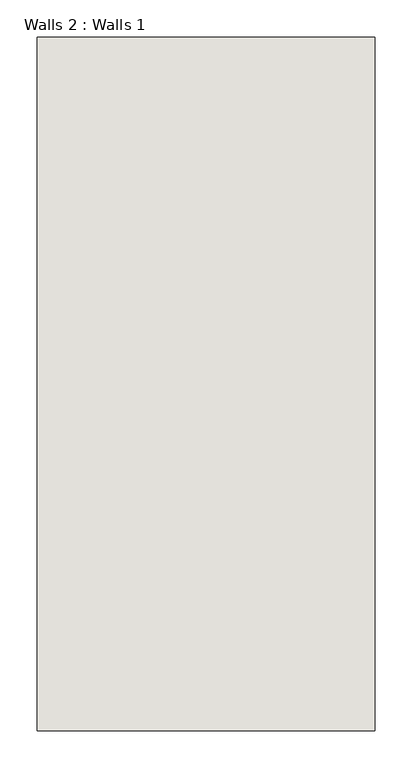
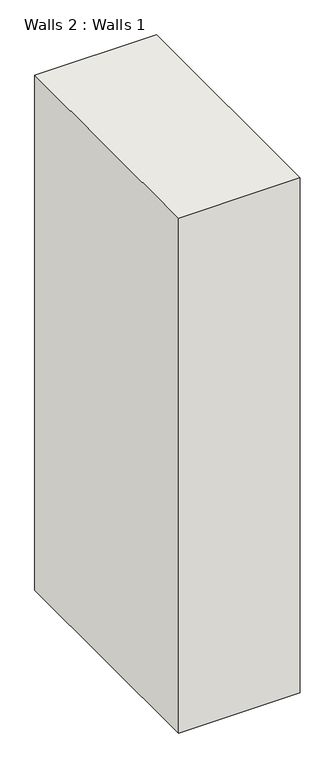
"""IFC4 building model written with IfcOpenShell, lengths in millimetres: wall geometry, Walls 2 : Walls 1."""

from ifc_helpers import new_model, si_unit, frame, origin, place, context, project, spatial, polyline, outline, extrude, faceted_brep, source, transform, mapped, element, save


def walls_2_walls_1_3d7729ba(model_context):
    return source(origin(), model_context, "Body", "SolidModel", [
        extrude(outline(polyline([(-8853.7371236, -1272.981648), (-8853.7371236, -2149.281648), (-9260.1371236, -2149.281648), (-9260.1371236, -1272.981648), (-8853.7371236, -1272.981648)])), frame((0.0, 0.0, 3775.1757913), z_axis=(0.0, 0.0, 1.0), x_axis=(1.0, 0.0, 0.0)), (0.0, 0.0, 1.0), 31.75),
        faceted_brep([(-8853.7371236, -1237.4497499, 5399.0952722), (-8853.7371236, -2174.681648, 5399.0952722), (-8853.7371236, -2174.681648, 3352.8), (-8853.7371236, -1237.4497499, 3352.8), (-8853.7371236, -1262.8497499, 5373.6952722), (-8853.7371236, -1262.8497499, 3378.2), (-8853.7371236, -2149.281648, 3378.2), (-8853.7371236, -2149.281648, 5373.6952722), (-9310.9371236, -1237.4497499, 5399.0952722), (-9310.9371236, -1237.4497499, 3352.8), (-9310.9371236, -2174.681648, 3352.8), (-9310.9371236, -2174.681648, 5399.0952722), (-9260.1371236, -1262.8497499, 5373.6952722), (-9260.1371236, -2149.281648, 5373.6952722), (-9260.1371236, -2149.281648, 3378.2), (-9260.1371236, -1262.8497499, 3378.2)], [[[0, 1, 2, 3], [4, 5, 6, 7]], [[8, 9, 10, 11]], [[1, 0, 8, 11]], [[2, 1, 11, 10]], [[3, 2, 10, 9]], [[0, 3, 9, 8]], [[12, 13, 14, 15]], [[12, 15, 5, 4]], [[15, 14, 6, 5]], [[14, 13, 7, 6]], [[13, 12, 4, 7]]]),
    ])


if __name__ == "__main__":
    model = new_model("IFC4")
    model_context = context("Model", 3, world=origin())
    ifc_project = project(units=[si_unit("LENGTHUNIT", "METRE", prefix="MILLI")], contexts=[model_context])
    site = spatial("IfcSite", under=ifc_project)
    building = spatial("IfcBuilding", under=site)
    placement = place(None, origin())
    walls_2_walls_1_shape = walls_2_walls_1_3d7729ba(model_context)
    element("IfcWall", 1, ObjectType="Walls 2 : Walls 1", at=placement, inside=building, context=model_context, shape_type="MappedRepresentation", body=[
        mapped(walls_2_walls_1_shape, transform((0.0, 0.0, 0.0), x_axis=(1.0, 0.0, 0.0), y_axis=(0.0, 1.0, 0.0), z_axis=(0.0, 0.0, 1.0))),
    ])
    save(model, "model.ifc")

# Revit data of these elements
# Element 1 (IfcWall, "Walls 2 : Walls 1")
#   Materials on its faces: "Default Wall"
# Materials
#   "Default Wall": colour RGB 128 128 128, transparency 0
